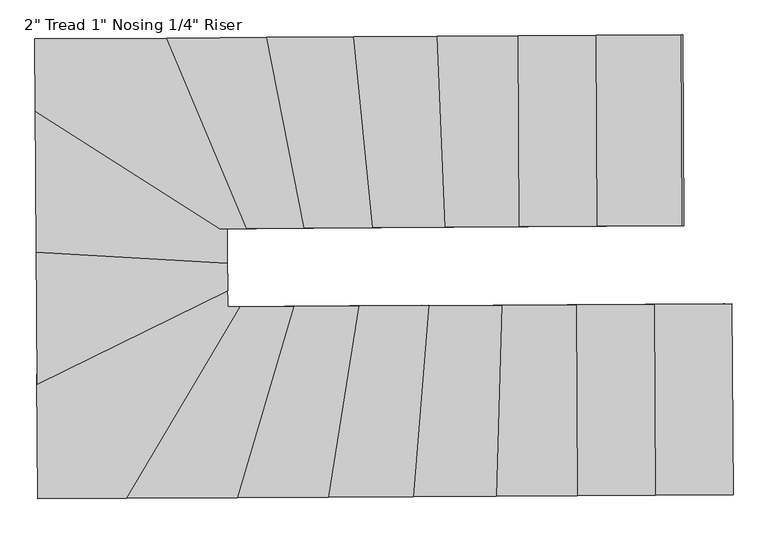
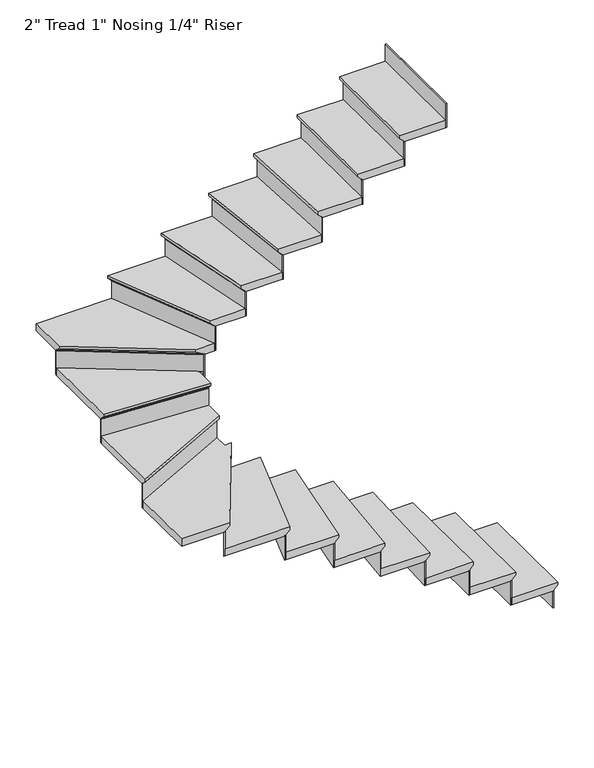
"""IFC4 building model written with IfcOpenShell, lengths in millimetres: stair flight geometry."""

from ifc_helpers import new_model, si_unit, origin, place, context, project, spatial, faceted_brep, source, transform, mapped, element, save


def stair_flight_03031656(model_context):
    return source(origin(), model_context, "Body", "Brep", [
        faceted_brep([(-120.6930289, -3539.621908, 150.2833333), (-120.6930289, -3539.621908, 169.3333333), (-116.4891496, -4225.4090232, 169.3333333), (-116.4891496, -4225.4090232, 150.2833333), (-146.0925517, -3539.7776072, 124.8833333), (-141.8886723, -4225.5647224, 124.8833333), (-425.4873024, -3541.4902988, 169.3333333), (-421.283423, -4227.277414, 169.3333333), (-141.8886723, -4225.5647224, 118.5333333), (-421.283423, -4227.277414, 118.5333333), (-425.4873024, -3541.4902988, 118.5333333), (-146.0925517, -3539.7776072, 118.5333333)], [[[0, 1, 2, 3]], [[4, 0, 3, 5]], [[2, 1, 6, 7]], [[8, 9, 10, 11]], [[2, 7, 9, 8, 5, 3]], [[8, 11, 4, 5]], [[6, 1, 0, 4, 11, 10]], [[7, 6, 10, 9]]]),
        faceted_brep([(-146.0925517, -3539.7776072, 118.5333333), (-146.0925517, -3539.7776072, 0.0), (-152.4424324, -3539.816532, 0.0), (-152.4424324, -3539.816532, 118.5333333), (-141.8886723, -4225.5647224, 118.5333333), (-148.238553, -4225.6036472, 118.5333333), (-148.238553, -4225.6036472, 0.0), (-141.8886723, -4225.5647224, 0.0)], [[[0, 1, 2, 3]], [[4, 5, 6, 7]], [[1, 0, 4, 7]], [[2, 1, 7, 6]], [[3, 2, 6, 5]], [[0, 3, 5, 4]]]),
        faceted_brep([(-425.4873024, -3541.4902988, 287.8666667), (-425.4873024, -3541.4902988, 118.5333333), (-431.8371831, -3541.5292236, 118.5333333), (-431.8371831, -3541.5292236, 287.8666667), (-421.283423, -4227.277414, 287.8666667), (-427.6333037, -4227.3163388, 287.8666667), (-427.6333037, -4227.3163388, 118.5333333), (-421.283423, -4227.277414, 118.5333333)], [[[0, 1, 2, 3]], [[4, 5, 6, 7]], [[1, 0, 4, 7]], [[2, 1, 7, 6]], [[3, 2, 6, 5]], [[0, 3, 5, 4]]]),
        faceted_brep([(-395.8839002, -4227.1217148, 338.6666667), (-400.0877796, -3541.3345996, 338.6666667), (-704.882053, -3543.2029904, 338.6666667), (-700.6781736, -4228.9901056, 338.6666667), (-421.283423, -4227.277414, 287.8666667), (-700.6781736, -4228.9901056, 287.8666667), (-704.882053, -3543.2029904, 287.8666667), (-425.4873024, -3541.4902988, 287.8666667), (-421.283423, -4227.277414, 294.2166667), (-395.8839002, -4227.1217148, 319.6166667), (-425.4873024, -3541.4902988, 294.2166667), (-400.0877796, -3541.3345996, 319.6166667)], [[[0, 1, 2, 3]], [[4, 5, 6, 7]], [[0, 3, 5, 4, 8, 9]], [[4, 7, 10, 8]], [[2, 1, 11, 10, 7, 6]], [[3, 2, 6, 5]], [[11, 1, 0, 9]], [[10, 11, 9, 8]]]),
        faceted_brep([(-704.882053, -3543.2029904, 457.2), (-704.882053, -3543.2029904, 287.8666667), (-711.2319337, -3543.2419152, 287.8666667), (-711.2319337, -3543.2419152, 457.2), (-700.6781736, -4228.9901056, 457.2), (-707.0280543, -4229.0290304, 457.2), (-707.0280543, -4229.0290304, 287.8666667), (-700.6781736, -4228.9901056, 287.8666667)], [[[0, 1, 2, 3]], [[4, 5, 6, 7]], [[1, 0, 4, 7]], [[2, 1, 7, 6]], [[3, 2, 6, 5]], [[0, 3, 5, 4]]]),
        faceted_brep([(-675.2786508, -4228.8344064, 508.0), (-679.4825302, -3543.0472912, 508.0), (-971.9344004, -3544.840023, 508.0), (-992.4483132, -4230.7786584, 508.0), (-700.6781736, -4228.9901056, 457.2), (-992.4483132, -4230.7786584, 457.2), (-971.9344004, -3544.840023, 457.2), (-704.882053, -3543.2029904, 457.2), (-700.6781736, -4228.9901056, 463.55), (-675.2786508, -4228.8344064, 488.95), (-704.882053, -3543.2029904, 463.55), (-679.4825302, -3543.0472912, 488.95)], [[[0, 1, 2, 3]], [[4, 5, 6, 7]], [[0, 3, 5, 4, 8, 9]], [[4, 7, 10, 8]], [[2, 1, 11, 10, 7, 6]], [[3, 2, 6, 5]], [[11, 1, 0, 9]], [[10, 11, 9, 8]]]),
        faceted_brep([(-971.9344004, -3544.840023, 626.5333333), (-971.9344004, -3544.840023, 457.2), (-978.2884043, -3544.8789731, 457.2), (-978.2884043, -3544.8789731, 626.5333333), (-992.4483132, -4230.7786584, 626.5333333), (-998.8023171, -4230.8176085, 626.5333333), (-998.8023171, -4230.8176085, 457.2), (-992.4483132, -4230.7786584, 457.2)], [[[0, 1, 2, 3]], [[4, 5, 6, 7]], [[1, 0, 4, 7]], [[2, 1, 7, 6]], [[3, 2, 6, 5]], [[0, 3, 5, 4]]]),
        faceted_brep([(-967.0322975, -4230.6228581, 677.3333333), (-946.5183848, -3544.6842227, 677.3333333), (-1233.842238, -3546.4455197, 677.3333333), (-1289.4900883, -4232.5995264, 677.3333333), (-992.4483132, -4230.7786584, 626.5333333), (-1289.4900883, -4232.5995264, 626.5333333), (-1233.842238, -3546.4455197, 626.5333333), (-971.9344004, -3544.840023, 626.5333333), (-992.4483132, -4230.7786584, 632.8833333), (-967.0322975, -4230.6228581, 658.2833333), (-971.9344004, -3544.840023, 632.8833333), (-946.5183848, -3544.6842227, 658.2833333)], [[[0, 1, 2, 3]], [[4, 5, 6, 7]], [[0, 3, 5, 4, 8, 9]], [[4, 7, 10, 8]], [[2, 1, 11, 10, 7, 6]], [[3, 2, 6, 5]], [[11, 1, 0, 9]], [[10, 11, 9, 8]]]),
        faceted_brep([(-1233.842238, -3546.4455197, 795.8666667), (-1233.842238, -3546.4455197, 626.5333333), (-1240.2162558, -3546.4845925, 626.5333333), (-1240.2162558, -3546.4845925, 795.8666667), (-1289.4900883, -4232.5995264, 795.8666667), (-1295.8641061, -4232.6385992, 795.8666667), (-1295.8641061, -4232.6385992, 626.5333333), (-1289.4900883, -4232.5995264, 626.5333333)], [[[0, 1, 2, 3]], [[4, 5, 6, 7]], [[1, 0, 4, 7]], [[2, 1, 7, 6]], [[3, 2, 6, 5]], [[0, 3, 5, 4]]]),
        faceted_brep([(-1263.994017, -4232.4432353, 846.6666667), (-1208.3461666, -3546.2892286, 846.6666667), (-1486.5415383, -3547.994568, 846.6666667), (-1596.081167, -4234.4789317, 846.6666667), (-1289.4900883, -4232.5995264, 795.8666667), (-1596.081167, -4234.4789317, 795.8666667), (-1486.5415383, -3547.994568, 795.8666667), (-1233.842238, -3546.4455197, 795.8666667), (-1289.4900883, -4232.5995264, 802.2166667), (-1263.994017, -4232.4432353, 827.6166667), (-1233.842238, -3546.4455197, 802.2166667), (-1208.3461666, -3546.2892286, 827.6166667)], [[[0, 1, 2, 3]], [[4, 5, 6, 7]], [[0, 3, 5, 4, 8, 9]], [[4, 7, 10, 8]], [[2, 1, 11, 10, 7, 6]], [[3, 2, 6, 5]], [[11, 1, 0, 9]], [[10, 11, 9, 8]]]),
        faceted_brep([(-1486.5415383, -3547.994568, 965.2), (-1486.5415383, -3547.994568, 795.8666667), (-1492.9781659, -3548.0340246, 795.8666667), (-1492.9781659, -3548.0340246, 965.2), (-1596.081167, -4234.4789317, 965.2), (-1602.5177946, -4234.5183882, 965.2), (-1602.5177946, -4234.5183882, 795.8666667), (-1596.081167, -4234.4789317, 795.8666667)], [[[0, 1, 2, 3]], [[4, 5, 6, 7]], [[1, 0, 4, 7]], [[2, 1, 7, 6]], [[3, 2, 6, 5]], [[0, 3, 5, 4]]]),
        faceted_brep([(-1570.3346568, -4234.3211054, 1016.0), (-1460.7950281, -3547.8367418, 1016.0), (-1720.1488607, -3549.4265824, 1016.0), (-1922.8306159, -4236.4819079, 1016.0), (-1596.081167, -4234.4789317, 965.2), (-1922.8306159, -4236.4819079, 965.2), (-1720.1488607, -3549.4265824, 965.2), (-1486.5415383, -3547.994568, 965.2), (-1596.081167, -4234.4789317, 971.55), (-1570.3346568, -4234.3211054, 996.95), (-1486.5415383, -3547.994568, 971.55), (-1460.7950281, -3547.8367418, 996.95)], [[[0, 1, 2, 3]], [[4, 5, 6, 7]], [[0, 3, 5, 4, 8, 9]], [[4, 7, 10, 8]], [[2, 1, 11, 10, 7, 6]], [[3, 2, 6, 5]], [[11, 1, 0, 9]], [[10, 11, 9, 8]]]),
        faceted_brep([(-1720.1488607, -3549.4265824, 1134.5333333), (-1720.1488607, -3549.4265824, 965.2), (-1726.781397, -3549.4672399, 965.2), (-1726.781397, -3549.4672399, 1134.5333333), (-1922.8306159, -4236.4819079, 1134.5333333), (-1929.4631522, -4236.5225654, 1134.5333333), (-1929.4631522, -4236.5225654, 965.2), (-1922.8306159, -4236.4819079, 965.2)], [[[0, 1, 2, 3]], [[4, 5, 6, 7]], [[1, 0, 4, 7]], [[2, 1, 7, 6]], [[3, 2, 6, 5]], [[0, 3, 5, 4]]]),
        faceted_brep([(-1896.3004707, -4236.3192779, 1185.3333333), (-1693.6187155, -3549.2639524, 1185.3333333), (-1917.3665941, -3550.6355283, 1185.3333333), (-2324.8688668, -4238.9464049, 1185.3333333), (-1922.8306159, -4236.4819079, 1134.5333333), (-2324.8688668, -4238.9464049, 1134.5333333), (-1917.3665941, -3550.6355283, 1134.5333333), (-1720.1488607, -3549.4265824, 1134.5333333), (-1922.8306159, -4236.4819079, 1140.8833333), (-1896.3004707, -4236.3192779, 1166.2833333), (-1720.1488607, -3549.4265824, 1140.8833333), (-1693.6187155, -3549.2639524, 1166.2833333)], [[[0, 1, 2, 3]], [[4, 5, 6, 7]], [[0, 3, 5, 4, 8, 9]], [[4, 7, 10, 8]], [[2, 1, 11, 10, 7, 6]], [[3, 2, 6, 5]], [[11, 1, 0, 9]], [[10, 11, 9, 8]]]),
        faceted_brep([(-1917.3665941, -3550.6355283, 1303.8666667), (-1917.3665941, -3550.6355283, 1134.5333333), (-1924.7728783, -3550.6809289, 1134.5333333), (-1924.7728783, -3550.6809289, 1303.8666667), (-2324.8688668, -4238.9464049, 1303.8666667), (-2332.275151, -4238.9918055, 1303.8666667), (-2332.275151, -4238.9918055, 1134.5333333), (-2324.8688668, -4238.9464049, 1134.5333333)], [[[0, 1, 2, 3]], [[4, 5, 6, 7]], [[1, 0, 4, 7]], [[2, 1, 7, 6]], [[3, 2, 6, 5]], [[0, 3, 5, 4]]]),
        faceted_brep([(-2615.3480869, -3801.2875551, 1354.6666667), (-2612.6544213, -4240.7105322, 1354.6666667), (-2295.24373, -4238.7648026, 1354.6666667), (-1887.7414574, -3550.4539261, 1354.6666667), (-1931.0711854, -3550.7195376, 1354.6666667), (-1931.5966592, -3464.9979706, 1354.6666667), (-2612.6544213, -4240.7105322, 1303.8666667), (-2615.3480869, -3801.2875551, 1303.8666667), (-1931.5966592, -3464.9979706, 1303.8666667), (-1931.0711854, -3550.7195376, 1303.8666667), (-1917.3665941, -3550.6355283, 1303.8666667), (-2324.8688668, -4238.9464049, 1303.8666667), (-1917.3665941, -3550.6355283, 1310.2166667), (-2324.8688668, -4238.9464049, 1310.2166667), (-1887.7414574, -3550.4539261, 1335.6166667), (-2295.24373, -4238.7648026, 1335.6166667)], [[[0, 1, 2, 3, 4, 5]], [[6, 7, 8, 9, 10, 11]], [[1, 0, 7, 6]], [[11, 10, 12, 13]], [[5, 4, 9, 8]], [[0, 5, 8, 7]], [[14, 3, 2, 15]], [[12, 14, 15, 13]], [[4, 3, 14, 12, 10, 9]], [[2, 1, 6, 11, 13, 15]]]),
        faceted_brep([(-1931.5966592, -3464.9979706, 1473.2), (-1931.5966592, -3464.9979706, 1303.8666667), (-1931.6399076, -3457.9427742, 1303.8666667), (-1931.6399076, -3457.9427742, 1473.2), (-2615.3480869, -3801.2875551, 1473.2), (-2615.3913353, -3794.2323587, 1473.2), (-2615.3913353, -3794.2323587, 1303.8666667), (-2615.3480869, -3801.2875551, 1303.8666667)], [[[0, 1, 2, 3]], [[4, 5, 6, 7]], [[1, 0, 4, 7]], [[2, 1, 7, 6]], [[3, 2, 6, 5]], [[0, 3, 5, 4]]]),
        faceted_brep([(-2615.1750933, -3829.5083406, 1524.0), (-1931.4236656, -3493.2187561, 1524.0), (-1932.1828972, -3369.3638122, 1524.0), (-2618.2387587, -3329.7265819, 1524.0), (-2615.3480869, -3801.2875551, 1473.2), (-2618.2387587, -3329.7265819, 1473.2), (-1932.1828972, -3369.3638122, 1473.2), (-1931.5966592, -3464.9979706, 1473.2), (-2615.3480869, -3801.2875551, 1479.55), (-2615.1750933, -3829.5083406, 1504.95), (-1931.5966592, -3464.9979706, 1479.55), (-1931.4236656, -3493.2187561, 1504.95)], [[[0, 1, 2, 3]], [[4, 5, 6, 7]], [[0, 3, 5, 4, 8, 9]], [[4, 7, 10, 8]], [[2, 1, 11, 10, 7, 6]], [[3, 2, 6, 5]], [[11, 1, 0, 9]], [[10, 11, 9, 8]]]),
        faceted_brep([(-1932.1828972, -3369.3638122, 1642.5333333), (-1932.1828972, -3369.3638122, 1473.2), (-1932.2219015, -3363.0009693, 1473.2), (-1932.2219015, -3363.0009693, 1642.5333333), (-2618.2387587, -3329.7265819, 1642.5333333), (-2618.277763, -3323.363739, 1642.5333333), (-2618.277763, -3323.363739, 1473.2), (-2618.2387587, -3329.7265819, 1473.2)], [[[0, 1, 2, 3]], [[4, 5, 6, 7]], [[1, 0, 4, 7]], [[2, 1, 7, 6]], [[3, 2, 6, 5]], [[0, 3, 5, 4]]]),
        faceted_brep([(-2618.0827416, -3355.1779533, 1693.3333333), (-1932.0268801, -3394.8151835, 1693.3333333), (-1932.783877, -3271.3247869, 1693.3333333), (-1912.0496222, -3271.1976858, 1693.3333333), (-2621.364296, -2819.8515342, 1693.3333333), (-2618.2387587, -3329.7265819, 1642.5333333), (-2621.364296, -2819.8515342, 1642.5333333), (-1912.0496222, -3271.1976858, 1642.5333333), (-1932.783877, -3271.3247869, 1642.5333333), (-1932.1828972, -3369.3638122, 1642.5333333), (-2618.2387587, -3329.7265819, 1648.8833333), (-2618.0827416, -3355.1779533, 1674.2833333), (-1932.1828972, -3369.3638122, 1648.8833333), (-1932.0268801, -3394.8151835, 1674.2833333)], [[[0, 1, 2, 3, 4]], [[5, 6, 7, 8, 9]], [[0, 4, 6, 5, 10, 11]], [[5, 9, 12, 10]], [[2, 1, 13, 12, 9, 8]], [[3, 2, 8, 7]], [[4, 3, 7, 6]], [[13, 1, 0, 11]], [[12, 13, 11, 10]]]),
        faceted_brep([(-1912.0496222, -3271.1976858, 1811.8666667), (-1912.0496222, -3271.1976858, 1642.5333333), (-1900.3341194, -3271.1258697, 1642.5333333), (-1900.3341194, -3271.1258697, 1811.8666667), (-2621.364296, -2819.8515342, 1811.8666667), (-2621.4106144, -2812.2955182, 1811.8666667), (-2621.4106144, -2812.2955182, 1642.5333333), (-2621.364296, -2819.8515342, 1642.5333333)], [[[0, 1, 2, 3]], [[4, 5, 6, 7]], [[1, 0, 4, 7]], [[2, 1, 7, 6]], [[3, 2, 6, 5]], [[0, 3, 5, 4]]]),
        faceted_brep([(-2121.4312205, -2586.6683113, 1862.6666667), (-2622.7748716, -2589.7415511, 1862.6666667), (-2621.1790223, -2850.0755978, 1862.6666667), (-1958.9116334, -3271.4849502, 1862.6666667), (-1835.3232791, -3270.7273529, 1862.6666667), (-2622.7748716, -2589.7415511, 1811.8666667), (-2121.4312205, -2586.6683113, 1811.8666667), (-1835.3232791, -3270.7273529, 1811.8666667), (-1912.0496222, -3271.1976858, 1811.8666667), (-2621.364296, -2819.8515342, 1811.8666667), (-2621.364296, -2819.8515342, 1818.2166667), (-2621.1790223, -2850.0755978, 1843.6166667), (-1912.0496222, -3271.1976858, 1818.2166667), (-1958.9116334, -3271.4849502, 1843.6166667)], [[[0, 1, 2, 3, 4]], [[5, 6, 7, 8, 9]], [[1, 0, 6, 5]], [[2, 1, 5, 9, 10, 11]], [[9, 8, 12, 10]], [[0, 4, 7, 6]], [[13, 3, 2, 11]], [[12, 13, 11, 10]], [[4, 3, 13, 12, 8, 7]]]),
        faceted_brep([(-1835.3232791, -3270.7273529, 1981.2), (-1835.3232791, -3270.7273529, 1811.8666667), (-1828.4578405, -3270.6852677, 1811.8666667), (-1828.4578405, -3270.6852677, 1981.2), (-2121.4312205, -2586.6683113, 1981.2), (-2114.5657819, -2586.6262261, 1981.2), (-2114.5657819, -2586.6262261, 1811.8666667), (-2121.4312205, -2586.6683113, 1811.8666667)], [[[0, 1, 2, 3]], [[4, 5, 6, 7]], [[1, 0, 4, 7]], [[2, 1, 7, 6]], [[3, 2, 6, 5]], [[0, 3, 5, 4]]]),
        faceted_brep([(-2148.8929752, -2586.8366521, 2032.0), (-1862.7850338, -3270.8956936, 2032.0), (-1630.6514822, -3269.4727134, 2032.0), (-1765.0751589, -2584.4838464, 2032.0), (-2121.4312205, -2586.6683113, 1981.2), (-1765.0751589, -2584.4838464, 1981.2), (-1630.6514822, -3269.4727134, 1981.2), (-1835.3232791, -3270.7273529, 1981.2), (-2121.4312205, -2586.6683113, 1987.55), (-2148.8929752, -2586.8366521, 2012.95), (-1835.3232791, -3270.7273529, 1987.55), (-1862.7850338, -3270.8956936, 2012.95)], [[[0, 1, 2, 3]], [[4, 5, 6, 7]], [[0, 3, 5, 4, 8, 9]], [[4, 7, 10, 8]], [[2, 1, 11, 10, 7, 6]], [[3, 2, 6, 5]], [[11, 1, 0, 9]], [[10, 11, 9, 8]]]),
        faceted_brep([(-1630.6514822, -3269.4727134, 2150.5333333), (-1630.6514822, -3269.4727134, 1981.2), (-1624.1881401, -3269.4330931, 1981.2), (-1624.1881401, -3269.4330931, 2150.5333333), (-1765.0751589, -2584.4838464, 2150.5333333), (-1758.6118168, -2584.4442261, 2150.5333333), (-1758.6118168, -2584.4442261, 1981.2), (-1765.0751589, -2584.4838464, 1981.2)], [[[0, 1, 2, 3]], [[4, 5, 6, 7]], [[1, 0, 4, 7]], [[2, 1, 7, 6]], [[3, 2, 6, 5]], [[0, 3, 5, 4]]]),
        faceted_brep([(-1790.9285273, -2584.6423277, 2201.3333333), (-1656.5048506, -3269.6311948, 2201.3333333), (-1385.319119, -3267.9688245, 2201.3333333), (-1452.3132293, -2582.5666138, 2201.3333333), (-1765.0751589, -2584.4838464, 2150.5333333), (-1452.3132293, -2582.5666138, 2150.5333333), (-1385.319119, -3267.9688245, 2150.5333333), (-1630.6514822, -3269.4727134, 2150.5333333), (-1765.0751589, -2584.4838464, 2156.8833333), (-1790.9285273, -2584.6423277, 2182.2833333), (-1630.6514822, -3269.4727134, 2156.8833333), (-1656.5048506, -3269.6311948, 2182.2833333)], [[[0, 1, 2, 3]], [[4, 5, 6, 7]], [[0, 3, 5, 4, 8, 9]], [[4, 7, 10, 8]], [[2, 1, 11, 10, 7, 6]], [[3, 2, 6, 5]], [[11, 1, 0, 9]], [[10, 11, 9, 8]]]),
        faceted_brep([(-1385.319119, -3267.9688245, 2319.8666667), (-1385.319119, -3267.9688245, 2150.5333333), (-1378.942678, -3267.9297369, 2150.5333333), (-1378.942678, -3267.9297369, 2319.8666667), (-1452.3132293, -2582.5666138, 2319.8666667), (-1445.9367882, -2582.5275262, 2319.8666667), (-1445.9367882, -2582.5275262, 2150.5333333), (-1452.3132293, -2582.5666138, 2150.5333333)], [[[0, 1, 2, 3]], [[4, 5, 6, 7]], [[1, 0, 4, 7]], [[2, 1, 7, 6]], [[3, 2, 6, 5]], [[0, 3, 5, 4]]]),
        faceted_brep([(-1477.8189934, -2582.7229643, 2370.6666667), (-1410.8248832, -3268.125175, 2370.6666667), (-1125.1141805, -3266.3737666, 2370.6666667), (-1153.9085026, -2580.7373909, 2370.6666667), (-1452.3132293, -2582.5666138, 2319.8666667), (-1153.9085026, -2580.7373909, 2319.8666667), (-1125.1141805, -3266.3737666, 2319.8666667), (-1385.319119, -3267.9688245, 2319.8666667), (-1452.3132293, -2582.5666138, 2326.2166667), (-1477.8189934, -2582.7229643, 2351.6166667), (-1385.319119, -3267.9688245, 2326.2166667), (-1410.8248832, -3268.125175, 2351.6166667)], [[[0, 1, 2, 3]], [[4, 5, 6, 7]], [[0, 3, 5, 4, 8, 9]], [[4, 7, 10, 8]], [[2, 1, 11, 10, 7, 6]], [[3, 2, 6, 5]], [[11, 1, 0, 9]], [[10, 11, 9, 8]]]),
        faceted_brep([(-1125.1141805, -3266.3737666, 2489.2), (-1125.1141805, -3266.3737666, 2319.8666667), (-1118.7602189, -3266.3348167, 2319.8666667), (-1118.7602189, -3266.3348167, 2489.2), (-1153.9085026, -2580.7373909, 2489.2), (-1147.554541, -2580.6984411, 2489.2), (-1147.554541, -2580.6984411, 2319.8666667), (-1153.9085026, -2580.7373909, 2319.8666667)], [[[0, 1, 2, 3]], [[4, 5, 6, 7]], [[1, 0, 4, 7]], [[2, 1, 7, 6]], [[3, 2, 6, 5]], [[0, 3, 5, 4]]]),
        faceted_brep([(-1179.3243487, -2580.8931902, 2540.0), (-1150.5300267, -3266.5295659, 2540.0), (-858.0309746, -3264.7365448, 2540.0), (-862.2348539, -2578.9494296, 2540.0), (-1153.9085026, -2580.7373909, 2489.2), (-862.2348539, -2578.9494296, 2489.2), (-858.0309746, -3264.7365448, 2489.2), (-1125.1141805, -3266.3737666, 2489.2), (-1153.9085026, -2580.7373909, 2495.55), (-1179.3243487, -2580.8931902, 2520.95), (-1125.1141805, -3266.3737666, 2495.55), (-1150.5300267, -3266.5295659, 2520.95)], [[[0, 1, 2, 3]], [[4, 5, 6, 7]], [[0, 3, 5, 4, 8, 9]], [[4, 7, 10, 8]], [[2, 1, 11, 10, 7, 6]], [[3, 2, 6, 5]], [[11, 1, 0, 9]], [[10, 11, 9, 8]]]),
        faceted_brep([(-858.0309746, -3264.7365448, 2658.5333333), (-858.0309746, -3264.7365448, 2489.2), (-851.6810939, -3264.69762, 2489.2), (-851.6810939, -3264.69762, 2658.5333333), (-862.2348539, -2578.9494296, 2658.5333333), (-855.8849733, -2578.9105048, 2658.5333333), (-855.8849733, -2578.9105048, 2489.2), (-862.2348539, -2578.9494296, 2489.2)], [[[0, 1, 2, 3]], [[4, 5, 6, 7]], [[1, 0, 4, 7]], [[2, 1, 7, 6]], [[3, 2, 6, 5]], [[0, 3, 5, 4]]]),
        faceted_brep([(-887.6343767, -2579.1051288, 2709.3333333), (-883.4304974, -3264.8922441, 2709.3333333), (-578.6362239, -3263.0238532, 2709.3333333), (-582.8401033, -2577.236738, 2709.3333333), (-862.2348539, -2578.9494296, 2658.5333333), (-582.8401033, -2577.236738, 2658.5333333), (-578.6362239, -3263.0238532, 2658.5333333), (-858.0309746, -3264.7365448, 2658.5333333), (-862.2348539, -2578.9494296, 2664.8833333), (-887.6343767, -2579.1051288, 2690.2833333), (-858.0309746, -3264.7365448, 2664.8833333), (-883.4304974, -3264.8922441, 2690.2833333)], [[[0, 1, 2, 3]], [[4, 5, 6, 7]], [[0, 3, 5, 4, 8, 9]], [[4, 7, 10, 8]], [[2, 1, 11, 10, 7, 6]], [[3, 2, 6, 5]], [[11, 1, 0, 9]], [[10, 11, 9, 8]]]),
        faceted_brep([(-578.6362239, -3263.0238532, 2827.8666667), (-578.6362239, -3263.0238532, 2658.5333333), (-572.2863432, -3262.9849284, 2658.5333333), (-572.2863432, -3262.9849284, 2827.8666667), (-582.8401033, -2577.236738, 2827.8666667), (-576.4902226, -2577.1978132, 2827.8666667), (-576.4902226, -2577.1978132, 2658.5333333), (-582.8401033, -2577.236738, 2658.5333333)], [[[0, 1, 2, 3]], [[4, 5, 6, 7]], [[1, 0, 4, 7]], [[2, 1, 7, 6]], [[3, 2, 6, 5]], [[0, 3, 5, 4]]]),
        faceted_brep([(-299.2414733, -3261.3111616, 2997.2), (-299.2414733, -3261.3111616, 2827.8666667), (-292.8915926, -3261.2722368, 2827.8666667), (-292.8915926, -3261.2722368, 2997.2), (-303.4453527, -2575.5240464, 2997.2), (-297.095472, -2575.4851216, 2997.2), (-297.095472, -2575.4851216, 2827.8666667), (-303.4453527, -2575.5240464, 2827.8666667)], [[[0, 1, 2, 3]], [[4, 5, 6, 7]], [[1, 0, 4, 7]], [[2, 1, 7, 6]], [[3, 2, 6, 5]], [[0, 3, 5, 4]]]),
        faceted_brep([(-608.2396261, -2577.3924372, 2878.6666667), (-604.0357467, -3263.1795525, 2878.6666667), (-299.2414733, -3261.3111616, 2878.6666667), (-303.4453527, -2575.5240464, 2878.6666667), (-582.8401033, -2577.236738, 2827.8666667), (-303.4453527, -2575.5240464, 2827.8666667), (-299.2414733, -3261.3111616, 2827.8666667), (-578.6362239, -3263.0238532, 2827.8666667), (-582.8401033, -2577.236738, 2834.2166667), (-608.2396261, -2577.3924372, 2859.6166667), (-578.6362239, -3263.0238532, 2834.2166667), (-604.0357467, -3263.1795525, 2859.6166667)], [[[0, 1, 2, 3]], [[4, 5, 6, 7]], [[0, 3, 5, 4, 8, 9]], [[4, 7, 10, 8]], [[2, 1, 11, 10, 7, 6]], [[3, 2, 6, 5]], [[11, 1, 0, 9]], [[10, 11, 9, 8]]]),
    ])


if __name__ == "__main__":
    model = new_model("IFC4")
    model_context = context("Model", 3, world=origin())
    ifc_project = project(units=[si_unit("LENGTHUNIT", "METRE", prefix="MILLI")], contexts=[model_context])
    site = spatial("IfcSite", under=ifc_project)
    building = spatial("IfcBuilding", under=site)
    placement = place(None, origin())
    stair_flight_shape = stair_flight_03031656(model_context)
    element("IfcStairFlight", 1, ObjectType="2\" Tread 1\" Nosing 1/4\" Riser", at=placement, inside=building, context=model_context, shape_type="MappedRepresentation", body=[
        mapped(stair_flight_shape, transform((0.0, 0.0, 0.0), x_axis=(1.0, 0.0, 0.0), y_axis=(0.0, 1.0, 0.0), z_axis=(0.0, 0.0, 1.0))),
    ])
    save(model, "model.ifc")
